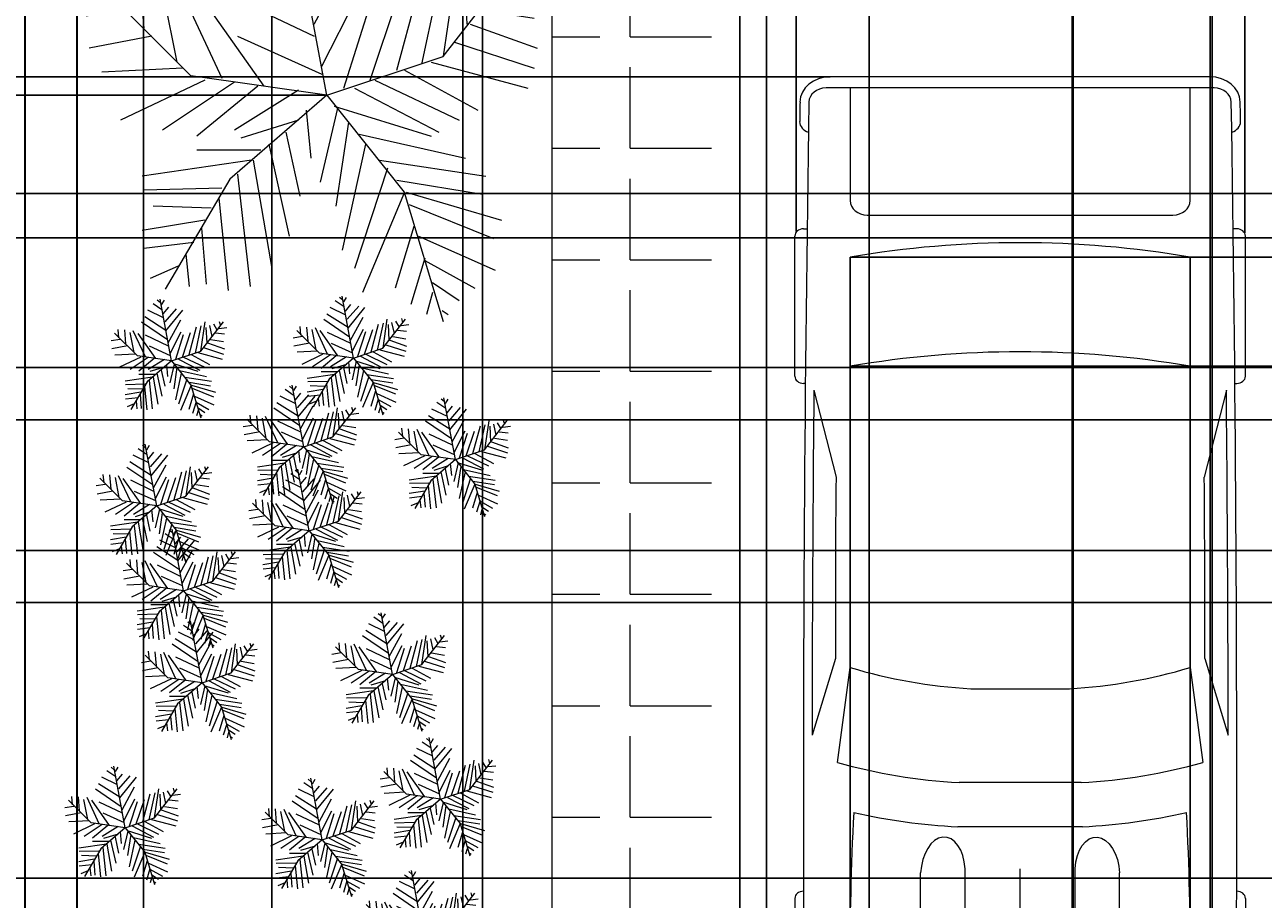
# Model space of a CAD drawing. Units: inches. Extents: x 818 to 1898, y 976 to 2364.
# Tile 4 of 96: x 993 to 1207, y 1295 to 1446. Entities that reach past the tile are written whole.
import ezdxf

# ---------------------------------------------------------------- set-up
doc = ezdxf.new("R2010")
doc.units = ezdxf.units.IN
doc.header["$LTSCALE"] = 5
doc.header["$MEASUREMENT"] = 0
for name, color, linetype, lineweight in [('A-ANNO-DIMS', 2, 'Continuous', 18), ('C-PKNG', 8, 'Continuous', 18), ('C-PKNG-PATT', 9, 'Continuous', 9), ('C-PROP', 7, 'Continuous', 35), ('L-PLNT-BEDS', 94, 'Continuous', 18)]:
    doc.layers.add(name, color=color, linetype=linetype, lineweight=lineweight)
doc.layers.add('L-PLNT', color=116, linetype='Continuous', lineweight=13, true_color=0x136734)
doc.styles.get("Standard").update_dxf_attribs({"font": 'arial.ttf'})
doc.dimstyles.get("Standard").update_dxf_attribs({"dimtxt": 0.18, "dimasz": 0.18, "dimexe": 0.18, "dimexo": 0.0625, "dimgap": 0.09, "dimtad": 0, "dimtih": 1, "dimtoh": 1, "dimdec": 4, "dimzin": 0, "dimdsep": 46, "dimtxsty": 'Standard', "dimcen": 0.09, "dimadec": 0, "dimazin": 0, "dimtfac": 1, "dimtdec": 4, "dimtofl": 0, "dimtmove": 0, "dimatfit": 3, "dimfxl": 1, "dimtolj": 1, "dimtzin": 0, "dimarcsym": 0})
pattern_1 = [(0, (0, 0), (0, 19.25), [14, -5.25]), (90, (0, 0), (-19.25, 1e-15), [14, -5.25])]

# ---------------------------------------------------------------- blocks, each defined once
blk = doc.blocks.new('*U13')
for p, q in [((46.55, 38.89), (22.35, 38.89)), ((136.7, 38.89), (160.9, 38.89)), ((47.8, 37.39), (47.8, 37.41)), ((135.45, 37.07), (135.45, 37.41)), ((162.15, 37.41), (162.15, 36.77)), ((87.99, 31.87), (74.76, 35.92)), ((134.31, 35.6), (119.29, 31.78)), ((186.47, -33.5), (186.47, 33.5)), ((188.4, -32.76), (188.4, 32.76)), ((70.03, 31.54), (86.41, 29.35)), ((138.42, 29.35), (157.25, 29.35)), ((186.47, 29.35), (167.01, 29.35)), ((164.52, 26.39), (164.52, -26.39)), ((36.13, 17.17), (50.94, 17.17)), ((58.92, -10.77), (58.92, 10.77)), ((29.77, 9.51), (51.68, 9.51)), ((66.55, -10.53), (66.55, 10.53)), ((186.47, -10.53), (186.47, 10.53)), ((82.74, 8.5), (82.74, -8.5)), ((0, 0), (51.68, 0)), ((29.77, -9.51), (51.68, -9.51)), ((36.13, -17.17), (50.94, -17.17)), ((86.41, -29.35), (70.03, -31.54)), ((157.25, -29.35), (138.42, -29.35)), ((167.01, -29.35), (186.47, -29.35)), ((87.99, -31.87), (74.76, -35.92)), ((134.31, -35.6), (119.29, -31.78)), ((47.8, -37.39), (47.8, -37.41)), ((135.45, -37.07), (135.45, -37.41)), ((162.15, -37.41), (162.15, -36.77)), ((46.55, -38.89), (22.35, -38.89)), ((136.7, -38.89), (160.9, -38.89))]:
    blk.add_line(p, q)
for centre, major_axis, ratio, start_param, end_param in [((46.55, 37.41), (0, 1.48), 0.842304, -1.570796, 0), ((136.7, 37.41), (0, -1.48), 0.842304, 3.141593, 4.712389), ((160.9, 37.41), (0, 1.48), 0.842304, -1.570796, 0), ((64.48, -10555.62), (0, 10593.03), 0.842304, -0.013397, 0.002797), ((180.63, 35.84), (0, 2.22), 0.842304, -0.013017, 1.249894), ((64.48, -10556.36), (0, 10595.31), 0.842304, -0.013397, -0.013017), ((183.98, 33.5), (0, -2.96), 0.842304, 1.570796, 3.128196), ((183.98, 32.76), (0, -5.25), 0.842304, 1.570796, 3.128196), ((64.48, -10555.62), (0, -10591.55), 0.842304, 3.133765, 3.140441), ((135.29, 5.39), (0, 81.77), 0.842304, 1.245306, 1.50788), ((95.79, -3666.35), (0, -3698.24), 0.842304, 3.134049, 3.144098), ((37.47, -593.96), (0, -623.33), 0.842304, 3.096046, 3.200911), ((134.4, 5.39), (0, -89.78), 0.842304, 4.449482, 4.652344), ((149.6, 2.8), (0, -79.58), 0.842304, 4.372215, 4.640744), ((17.08, 0), (0, 147.02), 0.842304, 4.511394, 4.913384), ((35.91, 0), (0, 147.02), 0.842304, 4.511394, 4.913384), ((167.01, 26.39), (0, 2.96), 0.842304, 0, 1.570796), ((50.79, 13.34), (6.34, -0.36), 0.603834, -1.395552, 1.581315), ((149.6, -2.8), (0, -79.58), 0.842304, -1.499151, -1.230623), ((135.29, -5.39), (0, -81.77), 0.842304, -1.50788, -1.245306), ((134.4, -5.39), (0, -89.78), 0.842304, -1.510751, -1.307889), ((167.01, -26.39), (0, -2.96), 0.842304, 4.712389, 6.283185), ((37.47, 593.96), (0, -623.33), 0.842304, -0.059319, 0.045547), ((95.79, 3666.35), (0, -3698.24), 0.842304, -0.002505, 0.007544), ((183.98, -33.5), (0, 2.96), 0.842304, 3.15499, 4.712389), ((183.98, -32.76), (0, -5.25), 0.842304, 0.013397, 1.570796), ((64.48, 10555.62), (0, -10591.55), 0.842304, 0.001152, 0.007828), ((64.48, 10555.62), (0, 10593.03), 0.842304, 3.138796, 3.15499), ((46.55, -37.41), (0, -1.48), 0.842304, 0, 1.570796), ((136.7, -37.41), (0, -1.48), 0.842304, -1.570796, 0), ((160.9, -37.41), (0, 1.48), 0.842304, 3.141593, 4.712389), ((180.63, -35.84), (0, -2.22), 0.842304, -1.249894, 0.013017), ((64.48, 10556.36), (0, 10595.31), 0.842304, 3.15461, 3.15499)]:
    blk.add_ellipse(centre, major_axis=major_axis, ratio=ratio, start_param=start_param, end_param=end_param)
at = {"extrusion": (0, 0, -1)}
blk.add_ellipse((50.79, -13.34), major_axis=(6.34, 0.36), ratio=0.603834, start_param=-1.395552, end_param=1.581315, dxfattribs=at)
blk = doc.blocks.new('SHRUB-ACCENT')
for p, q in [((8.8, 18.63), (7.25, 19.67)), ((8.53, 19.84), (7.99, 20.28)), ((10.44, 9.82), (8.47, 20.47)), ((8.74, 19.5), (9.21, 20.28)), ((9.48, 15.07), (5.82, 17.41)), ((9.08, 17.24), (6.37, 18.54)), ((9.01, 17.93), (9.96, 19.06)), ((9.35, 16.54), (11.31, 18.8)), ((9.48, 14.98), (12.39, 18.54)), ((1.35, 13.77), (1.22, 15.24)), ((2.3, 15.16), (2.51, 12.72)), ((3.79, 15.07), (5.89, 10.55)), ((9.75, 13.42), (5.28, 16.46)), ((9.89, 12.9), (12.06, 16.89)), ((13.48, 10.9), (14.76, 15.68)), ((14.56, 11.16), (15.58, 15.85)), ((15.49, 11.5), (19.41, 16.55)), ((15.51, 11.51), (16.25, 16.54)), ((16.39, 15.59), (16.53, 12.9)), ((17, 15.94), (17.41, 14.03)), ((17.68, 16.2), (18.29, 15.16)), ((18.62, 15.42), (19.98, 15.59)), ((18.69, 16.63), (18.9, 15.94)), ((1.56, 13.51), (0, 13.25)), ((4.55, 10.66), (0.62, 14.58)), ((3.25, 14.72), (3.93, 11.25)), ((7.72, 10.21), (4.67, 14.55)), ((5.89, 14.29), (9.89, 12.38)), ((10.23, 11.07), (12.12, 14.81)), ((11.17, 10.12), (12.53, 14.37)), ((12.33, 10.47), (13.75, 14.72)), ((16.66, 12.9), (19.57, 11.86)), ((17.2, 13.51), (19.44, 13.16)), ((18.02, 14.63), (19.57, 14.46)), ((2.84, 12.38), (0.14, 11.86)), ((4.2, 10.99), (0.68, 10.81)), ((6.57, 12.38), (10.23, 10.73)), ((10.44, 9.82), (15.49, 11.5)), ((13.82, 10.9), (17, 9.16)), ((14.97, 11.25), (19.17, 10.12)), ((15.98, 12.12), (19.44, 10.99)), ((5.15, 10.47), (1.49, 8.73)), ((6.43, 10.38), (3.32, 8.3)), ((10.44, 9.82), (4.55, 10.66)), ((7.45, 10.21), (4.81, 8.04)), ((10.44, 9.82), (6.23, 6.17)), ((9.21, 10.03), (6.43, 8.3)), ((9.21, 8.73), (6.7, 7.95)), ((9.55, 9.16), (9.75, 7.08)), ((10.9, 9.25), (10.16, 6.04)), ((10.44, 9.82), (13.8, 5.61)), ((10.77, 9.34), (14.97, 8.04)), ((11.38, 8.64), (10.84, 5)), ((11.65, 10.12), (15.31, 8.21)), ((12.53, 10.47), (16.19, 8.73)), ((7.18, 6.99), (2.44, 6.3)), ((7.59, 7.43), (4.81, 7.43)), ((7.25, 6.99), (8.06, 2.31)), ((7.92, 7.69), (8.8, 3.69)), ((8.67, 8.21), (9.28, 5.43)), ((12.12, 7.69), (11.11, 3.09)), ((13.07, 6.65), (11.65, 2.31)), ((11.85, 8.12), (16.46, 7.08)), ((12.73, 6.99), (17.34, 6.3)), ((5.15, 4.39), (2.44, 3.95)), ((5.89, 5.78), (2.51, 5.69)), ((5.42, 4.91), (2.91, 5)), ((6.23, 6.17), (3.43, 1.4)), ((5.76, 5.34), (6.16, 1.35)), ((6.57, 6.39), (7.11, 1.52)), ((13.82, 5.6), (11.99, 1.26)), ((13.48, 6.13), (17.2, 5.52)), ((13.8, 5.61), (15.49, 0)), ((13.88, 5.6), (18.02, 4.39)), ((14.02, 5.08), (17.68, 3.61)), ((4.67, 3.43), (2.51, 3.17)), ((4, 2.39), (2.78, 1.87)), ((4.33, 2.91), (4.47, 1.52)), ((5.01, 4.04), (5.21, 1.61)), ((14.22, 4.13), (13.41, 1.44)), ((14.7, 2.74), (14.09, 0.74)), ((14.43, 3.69), (17.74, 2.22)), ((14.7, 2.65), (16.86, 1.44)), ((15.04, 1.26), (14.76, 0.31)), ((15.04, 1.7), (16.19, 0.92)), ((15.44, 0.48), (15.71, 0.31))]:
    blk.add_line(p, q)
blk = doc.blocks.new('PALM-BORDER')
for p, q in [((41.53, 39.05), (33.72, 81.45)), ((33.95, 78.95), (31.8, 80.68)), ((34.76, 77.57), (36.65, 80.68)), ((35.03, 74.11), (28.83, 78.26)), ((35.84, 71.35), (39.61, 75.84)), ((36.11, 68.59), (25.33, 73.77)), ((37.18, 65.82), (45, 74.8)), ((37.72, 59.6), (49.31, 73.77)), ((37.72, 59.95), (23.17, 69.28)), ((39.34, 51.31), (47.96, 67.2)), ((38.8, 53.39), (21.02, 65.48)), ((61.61, 45.75), (77.23, 65.83)), ((61.71, 45.79), (64.67, 65.82)), ((70.33, 64.44), (72.75, 60.3)), ((74.37, 66.17), (75.18, 63.4)), ((53.62, 43.37), (58.74, 62.37)), ((57.93, 44.41), (61.97, 63.06)), ((65.21, 62.02), (65.75, 51.31)), ((67.63, 63.4), (69.25, 55.81)), ((74.1, 61.33), (79.49, 62.02)), ((5.39, 54.77), (4.85, 60.64)), ((9.16, 60.3), (9.97, 50.62)), ((15.09, 59.95), (23.44, 41.99)), ((18.1, 42.4), (2.48, 58.02)), ((12.93, 58.57), (15.63, 44.75)), ((30.72, 40.61), (18.59, 57.88)), ((40.69, 44.06), (48.23, 58.91)), ((49.04, 41.64), (54.7, 58.57)), ((71.68, 58.22), (77.87, 57.53)), ((23.44, 56.84), (39.34, 49.24)), ((44.46, 40.26), (49.85, 57.19)), ((6.2, 53.73), (0, 52.7)), ((68.44, 53.73), (77.33, 52.35)), ((66.29, 51.31), (77.87, 47.17)), ((11.32, 49.24), (0.54, 47.17)), ((26.14, 49.24), (40.69, 42.68)), ((63.59, 48.21), (77.33, 43.71)), ((41.53, 39.05), (61.61, 45.75)), ((16.71, 43.71), (2.69, 43.02)), ((54.97, 43.37), (67.63, 36.46)), ((59.55, 44.75), (76.26, 40.26)), ((20.48, 41.64), (5.93, 34.73)), ((25.6, 41.3), (13.2, 33.01)), ((41.53, 39.05), (18.1, 42.4)), ((49.85, 41.64), (64.4, 34.73)), ((29.64, 40.61), (19.13, 31.97)), ((41.53, 39.05), (24.79, 24.55)), ((36.65, 39.91), (25.6, 33.01)), ((41.53, 39.05), (54.92, 22.32)), ((46.35, 40.26), (60.9, 32.66)), ((37.99, 36.46), (38.8, 28.17)), ((43.38, 36.81), (40.42, 24.02)), ((42.84, 37.15), (59.55, 31.97)), ((36.65, 34.73), (26.68, 31.62)), ((45.27, 34.39), (43.11, 19.88)), ((34.49, 32.66), (36.92, 21.61)), ((47.15, 32.32), (65.48, 28.17)), ((31.53, 30.59), (35.03, 14.7)), ((48.23, 30.59), (44.19, 12.28)), ((28.56, 27.82), (9.7, 25.06)), ((30.18, 29.55), (19.13, 29.55)), ((28.83, 27.82), (32.07, 9.17)), ((50.66, 27.82), (68.98, 25.06)), ((52, 26.44), (46.35, 9.17)), ((24.79, 24.55), (13.63, 5.58)), ((26.14, 25.41), (28.29, 6.06)), ((53.62, 24.37), (68.44, 21.95)), ((23.44, 22.99), (9.97, 22.64)), ((54.97, 22.3), (47.69, 5.02)), ((54.92, 22.32), (61.61, 0)), ((55.24, 22.3), (71.68, 17.46)), ((21.56, 19.53), (11.59, 19.88)), ((22.9, 21.26), (24.52, 5.37)), ((55.78, 20.22), (70.33, 14.35)), ((20.48, 17.46), (9.7, 15.73)), ((19.94, 16.08), (20.75, 6.41)), ((56.59, 16.42), (53.35, 5.72)), ((18.59, 13.66), (9.97, 12.62)), ((57.39, 14.7), (70.6, 8.83)), ((17.24, 11.59), (17.78, 6.06)), ((58.47, 10.9), (56.05, 2.95)), ((15.9, 9.52), (11.05, 7.44)), ((58.47, 10.55), (67.09, 5.72)), ((59.82, 6.75), (64.4, 3.64)), ((59.82, 5.02), (58.74, 1.22)), ((61.44, 1.92), (62.51, 1.22))]:
    blk.add_line(p, q)
blk = doc.blocks.new('*D59')
at = {"layer": 'A-ANNO-DIMS', "color": 0, "lineweight": -2, "ltscale": 5, "transparency": 16777216}
for p, q in [((1251.64, 2300.39), (818.03, 2300.39)), ((818.21, 2300.21), (818.21, 1669.95)), ((818.21, 1039.32), (818.21, 1669.59)), ((896.05, 1039.14), (818.03, 1039.14))]:
    blk.add_line(p, q, dxfattribs=at)
at = {"layer": 'A-ANNO-DIMS', "color": 0, "ltscale": 5, "transparency": 16777216}
for points in [[(818.18, 2300.21), (818.24, 2300.21), (818.21, 2300.39)], [(818.18, 1039.32), (818.24, 1039.32), (818.21, 1039.14)]]:
    blk.add_solid(points, dxfattribs=at)
at = {"layer": 'Defpoints', "color": 0, "ltscale": 5, "transparency": 16777216}
for p in [(818.21, 2300.39), (1251.71, 2300.39), (896.11, 1039.14)]:
    blk.add_point(p, dxfattribs=at)
at = {"layer": 'A-ANNO-DIMS', "color": 0, "ltscale": 5, "transparency": 16777216, "insert": (818.21, 1669.77), "char_height": 0.18, "attachment_point": 5}
blk.add_mtext('\\A1;1261.2', dxfattribs=at)
blk = doc.blocks.new('*D61')
at = {"layer": 'A-ANNO-DIMS', "color": 0, "lineweight": -2, "ltscale": 5, "transparency": 16777216}
for p, q in [((1071.73, 1203.03), (1071.73, 2363.87)), ((1071.91, 2363.69), (1250.94, 2363.69)), ((1430.55, 2363.69), (1251.51, 2363.69)), ((1430.73, 1203.03), (1430.73, 2363.87))]:
    blk.add_line(p, q, dxfattribs=at)
at = {"layer": 'A-ANNO-DIMS', "color": 0, "ltscale": 5, "transparency": 16777216}
for points in [[(1071.91, 2363.72), (1071.91, 2363.66), (1071.73, 2363.69)], [(1430.55, 2363.72), (1430.55, 2363.66), (1430.73, 2363.69)]]:
    blk.add_solid(points, dxfattribs=at)
at = {"layer": 'Defpoints', "color": 0, "ltscale": 5, "transparency": 16777216}
for p in [(1430.73, 2363.69), (1071.73, 1202.96), (1430.73, 1202.96)]:
    blk.add_point(p, dxfattribs=at)
at = {"layer": 'A-ANNO-DIMS', "color": 0, "ltscale": 5, "transparency": 16777216, "insert": (1251.23, 2363.69), "char_height": 0.18, "attachment_point": 5}
blk.add_mtext('\\A1;359', dxfattribs=at)
blk = doc.blocks.new('*D63')
at = {"layer": 'A-ANNO-DIMS', "color": 0, "lineweight": -2, "ltscale": 5, "transparency": 16777216}
for p, q in [((1116.13, 1485.2), (818.03, 1485.2)), ((818.21, 1485.02), (818.21, 1360.77)), ((818.21, 1236.14), (818.21, 1360.4)), ((1116.13, 1235.96), (818.03, 1235.96))]:
    blk.add_line(p, q, dxfattribs=at)
at = {"layer": 'A-ANNO-DIMS', "color": 0, "ltscale": 5, "transparency": 16777216}
for points in [[(818.18, 1485.02), (818.24, 1485.02), (818.21, 1485.2)], [(818.18, 1236.14), (818.24, 1236.14), (818.21, 1235.96)]]:
    blk.add_solid(points, dxfattribs=at)
at = {"layer": 'Defpoints', "color": 0, "ltscale": 5, "transparency": 16777216}
for p in [(818.21, 1485.2), (1116.19, 1485.2), (1116.19, 1235.96)]:
    blk.add_point(p, dxfattribs=at)
at = {"layer": 'A-ANNO-DIMS', "color": 0, "ltscale": 5, "transparency": 16777216, "insert": (818.21, 1360.58), "char_height": 0.18, "attachment_point": 5}
blk.add_mtext('\\A1;249.24', dxfattribs=at)
blk = doc.blocks.new('*D79')
at = {"layer": 'A-ANNO-DIMS', "color": 0, "lineweight": -2, "ltscale": 5, "transparency": 16777216}
for p, q in [((992.73, 1203.03), (992.73, 2363.87)), ((992.91, 2363.69), (1032.01, 2363.69)), ((1071.55, 2363.69), (1032.44, 2363.69)), ((1071.73, 1203.03), (1071.73, 2363.87))]:
    blk.add_line(p, q, dxfattribs=at)
at = {"layer": 'A-ANNO-DIMS', "color": 0, "ltscale": 5, "transparency": 16777216}
for points in [[(992.91, 2363.72), (992.91, 2363.66), (992.73, 2363.69)], [(1071.55, 2363.72), (1071.55, 2363.66), (1071.73, 2363.69)]]:
    blk.add_solid(points, dxfattribs=at)
at = {"layer": 'Defpoints', "color": 0, "ltscale": 5, "transparency": 16777216}
for p in [(1071.73, 2363.69), (992.73, 1202.96), (1071.73, 1202.96)]:
    blk.add_point(p, dxfattribs=at)
at = {"layer": 'A-ANNO-DIMS', "color": 0, "ltscale": 5, "transparency": 16777216, "insert": (1032.23, 2363.69), "char_height": 0.18, "attachment_point": 5}
blk.add_mtext('\\A1;79', dxfattribs=at)
blk = doc.blocks.new('*D91')
at = {"layer": 'A-ANNO-DIMS', "color": 0, "lineweight": -2, "ltscale": 5, "transparency": 16777216}
for p, q in [((959.17, 1071.12), (959.17, 2363.87)), ((959.35, 2363.69), (985.8, 2363.69)), ((1013.04, 2363.69), (986.59, 2363.69)), ((1013.22, 1071.12), (1013.22, 2363.87))]:
    blk.add_line(p, q, dxfattribs=at)
at = {"layer": 'A-ANNO-DIMS', "color": 0, "ltscale": 5, "transparency": 16777216}
for points in [[(959.35, 2363.72), (959.35, 2363.66), (959.17, 2363.69)], [(1013.04, 2363.72), (1013.04, 2363.66), (1013.22, 2363.69)]]:
    blk.add_solid(points, dxfattribs=at)
at = {"layer": 'Defpoints', "color": 0, "ltscale": 5, "transparency": 16777216}
for p in [(1013.22, 2363.69), (959.17, 1071.06), (1013.22, 1071.06)]:
    blk.add_point(p, dxfattribs=at)
at = {"layer": 'A-ANNO-DIMS', "color": 0, "ltscale": 5, "transparency": 16777216, "insert": (986.2, 2363.69), "char_height": 0.18, "attachment_point": 5}
blk.add_mtext('\\A1;54.04', dxfattribs=at)
blk = doc.blocks.new('*D92')
at = {"layer": 'A-ANNO-DIMS', "color": 0, "lineweight": -2, "ltscale": 5, "transparency": 16777216}
for p, q in [((1013.22, 1071.12), (1013.22, 2363.87)), ((1013.4, 2363.69), (1040.38, 2363.69)), ((1068.16, 2363.69), (1041.17, 2363.69)), ((1068.34, 1071.12), (1068.34, 2363.87))]:
    blk.add_line(p, q, dxfattribs=at)
at = {"layer": 'A-ANNO-DIMS', "color": 0, "ltscale": 5, "transparency": 16777216}
for points in [[(1013.4, 2363.72), (1013.4, 2363.66), (1013.22, 2363.69)], [(1068.16, 2363.72), (1068.16, 2363.66), (1068.34, 2363.69)]]:
    blk.add_solid(points, dxfattribs=at)
at = {"layer": 'Defpoints', "color": 0, "ltscale": 5, "transparency": 16777216}
for p in [(1068.34, 2363.69), (1013.22, 1071.06), (1068.34, 1071.06)]:
    blk.add_point(p, dxfattribs=at)
at = {"layer": 'A-ANNO-DIMS', "color": 0, "ltscale": 5, "transparency": 16777216, "insert": (1040.78, 2363.69), "char_height": 0.18, "attachment_point": 5}
blk.add_mtext('\\A1;55.12', dxfattribs=at)
blk = doc.blocks.new('*D93')
at = {"layer": 'A-ANNO-DIMS', "color": 0, "lineweight": -2, "ltscale": 5, "transparency": 16777216}
for p, q in [((1068.34, 1071.12), (1068.34, 2363.87)), ((1068.52, 2363.69), (1094.16, 2363.69)), ((1120.58, 2363.69), (1094.94, 2363.69)), ((1120.76, 1071.12), (1120.76, 2363.87))]:
    blk.add_line(p, q, dxfattribs=at)
at = {"layer": 'A-ANNO-DIMS', "color": 0, "ltscale": 5, "transparency": 16777216}
for points in [[(1068.52, 2363.72), (1068.52, 2363.66), (1068.34, 2363.69)], [(1120.58, 2363.72), (1120.58, 2363.66), (1120.76, 2363.69)]]:
    blk.add_solid(points, dxfattribs=at)
at = {"layer": 'Defpoints', "color": 0, "ltscale": 5, "transparency": 16777216}
for p in [(1120.76, 2363.69), (1068.34, 1071.06), (1120.76, 1071.06)]:
    blk.add_point(p, dxfattribs=at)
at = {"layer": 'A-ANNO-DIMS', "color": 0, "ltscale": 5, "transparency": 16777216, "insert": (1094.55, 2363.69), "char_height": 0.18, "attachment_point": 5}
blk.add_mtext('\\A1;52.42', dxfattribs=at)
blk = doc.blocks.new('*D94')
at = {"layer": 'A-ANNO-DIMS', "color": 0, "lineweight": -2, "ltscale": 5, "transparency": 16777216}
for p, q in [((1120.76, 1071.12), (1120.76, 2363.87)), ((1120.94, 2363.69), (1146.76, 2363.69)), ((1173.36, 2363.69), (1147.55, 2363.69)), ((1173.54, 1071.12), (1173.54, 2363.87))]:
    blk.add_line(p, q, dxfattribs=at)
at = {"layer": 'A-ANNO-DIMS', "color": 0, "ltscale": 5, "transparency": 16777216}
for points in [[(1120.94, 2363.72), (1120.94, 2363.66), (1120.76, 2363.69)], [(1173.36, 2363.72), (1173.36, 2363.66), (1173.54, 2363.69)]]:
    blk.add_solid(points, dxfattribs=at)
at = {"layer": 'Defpoints', "color": 0, "ltscale": 5, "transparency": 16777216}
for p in [(1173.54, 2363.69), (1120.76, 1071.06), (1173.54, 1071.06)]:
    blk.add_point(p, dxfattribs=at)
at = {"layer": 'A-ANNO-DIMS', "color": 0, "ltscale": 5, "transparency": 16777216, "insert": (1147.15, 2363.69), "char_height": 0.18, "attachment_point": 5}
blk.add_mtext('\\A1;52.78', dxfattribs=at)
blk = doc.blocks.new('*D95')
at = {"layer": 'A-ANNO-DIMS', "color": 0, "lineweight": -2, "ltscale": 5, "transparency": 16777216}
for p, q in [((1173.54, 1071.12), (1173.54, 2363.87)), ((1173.72, 2363.69), (1201.29, 2363.69)), ((1229.47, 2363.69), (1201.9, 2363.69)), ((1229.65, 1071.12), (1229.65, 2363.87))]:
    blk.add_line(p, q, dxfattribs=at)
at = {"layer": 'A-ANNO-DIMS', "color": 0, "ltscale": 5, "transparency": 16777216}
for points in [[(1173.72, 2363.72), (1173.72, 2363.66), (1173.54, 2363.69)], [(1229.47, 2363.72), (1229.47, 2363.66), (1229.65, 2363.69)]]:
    blk.add_solid(points, dxfattribs=at)
at = {"layer": 'Defpoints', "color": 0, "ltscale": 5, "transparency": 16777216}
for p in [(1229.65, 2363.69), (1173.54, 1071.06), (1229.65, 1071.06)]:
    blk.add_point(p, dxfattribs=at)
at = {"layer": 'A-ANNO-DIMS', "color": 0, "ltscale": 5, "transparency": 16777216, "insert": (1201.59, 2363.69), "char_height": 0.18, "attachment_point": 5}
blk.add_mtext('\\A1;56.1', dxfattribs=at)
blk = doc.blocks.new('*D108')
at = {"layer": 'A-ANNO-DIMS', "color": 0, "lineweight": -2, "ltscale": 5, "transparency": 16777216}
for p, q in [((1131.74, 1436.86), (818.03, 1436.86)), ((818.21, 1436.68), (818.21, 1342.84)), ((818.21, 1248.64), (818.21, 1342.48)), ((1164.49, 1248.46), (818.03, 1248.46))]:
    blk.add_line(p, q, dxfattribs=at)
at = {"layer": 'A-ANNO-DIMS', "color": 0, "ltscale": 5, "transparency": 16777216}
for points in [[(818.18, 1436.68), (818.24, 1436.68), (818.21, 1436.86)], [(818.18, 1248.64), (818.24, 1248.64), (818.21, 1248.46)]]:
    blk.add_solid(points, dxfattribs=at)
at = {"layer": 'Defpoints', "color": 0, "ltscale": 5, "transparency": 16777216}
for p in [(818.21, 1436.86), (1131.8, 1436.86), (1164.56, 1248.46)]:
    blk.add_point(p, dxfattribs=at)
at = {"layer": 'A-ANNO-DIMS', "color": 0, "ltscale": 5, "transparency": 16777216, "insert": (818.21, 1342.66), "char_height": 0.18, "attachment_point": 5}
blk.add_mtext('\\A1;188.4', dxfattribs=at)
blk = doc.blocks.new('*D109')
at = {"layer": 'A-ANNO-DIMS', "color": 0, "lineweight": -2, "ltscale": 5, "transparency": 16777216}
for p, q in [((1125.92, 1410.12), (1125.92, 2363.87)), ((1126.1, 2363.69), (1164.25, 2363.69)), ((1203.15, 2363.69), (1165, 2363.69)), ((1203.33, 1409.91), (1203.33, 2363.87))]:
    blk.add_line(p, q, dxfattribs=at)
at = {"layer": 'A-ANNO-DIMS', "color": 0, "ltscale": 5, "transparency": 16777216}
for points in [[(1126.1, 2363.72), (1126.1, 2363.66), (1125.92, 2363.69)], [(1203.15, 2363.72), (1203.15, 2363.66), (1203.33, 2363.69)]]:
    blk.add_solid(points, dxfattribs=at)
at = {"layer": 'Defpoints', "color": 0, "ltscale": 5, "transparency": 16777216}
for p in [(1203.33, 2363.69), (1125.92, 1410.05), (1203.33, 1409.85)]:
    blk.add_point(p, dxfattribs=at)
at = {"layer": 'A-ANNO-DIMS', "color": 0, "ltscale": 5, "transparency": 16777216, "insert": (1164.62, 2363.69), "char_height": 0.18, "attachment_point": 5}
blk.add_mtext('\\A1;77.41', dxfattribs=at)
blk = doc.blocks.new('*D111')
at = {"layer": 'A-ANNO-DIMS', "color": 0, "lineweight": -2, "ltscale": 5, "transparency": 16777216}
for p, q in [((1135.21, 1405.65), (1135.21, 975.66)), ((1193.91, 1405.65), (1193.91, 975.66)), ((1135.39, 975.84), (1164.23, 975.84)), ((1193.73, 975.84), (1164.88, 975.84))]:
    blk.add_line(p, q, dxfattribs=at)
at = {"layer": 'A-ANNO-DIMS', "color": 0, "ltscale": 5, "transparency": 16777216}
for points in [[(1135.39, 975.87), (1135.39, 975.81), (1135.21, 975.84)], [(1193.73, 975.87), (1193.73, 975.81), (1193.91, 975.84)]]:
    blk.add_solid(points, dxfattribs=at)
at = {"layer": 'Defpoints', "color": 0, "ltscale": 5, "transparency": 16777216}
for p in [(1135.21, 1405.71), (1193.91, 1405.71), (1193.91, 975.84)]:
    blk.add_point(p, dxfattribs=at)
at = {"layer": 'A-ANNO-DIMS', "color": 0, "ltscale": 5, "transparency": 16777216, "insert": (1164.56, 975.84), "char_height": 0.18, "attachment_point": 5}
blk.add_mtext('\\A1;58.7', dxfattribs=at)
blk = doc.blocks.new('*D112')
at = {"layer": 'A-ANNO-DIMS', "color": 0, "lineweight": -2, "ltscale": 5, "transparency": 16777216}
for p, q in [((1135.27, 1405.71), (1897.92, 1405.71)), ((1897.74, 1405.53), (1897.74, 1396.48)), ((1897.74, 1387.07), (1897.74, 1396.12)), ((1135.27, 1386.89), (1897.92, 1386.89))]:
    blk.add_line(p, q, dxfattribs=at)
at = {"layer": 'A-ANNO-DIMS', "color": 0, "ltscale": 5, "transparency": 16777216}
for points in [[(1897.71, 1405.53), (1897.77, 1405.53), (1897.74, 1405.71)], [(1897.71, 1387.07), (1897.77, 1387.07), (1897.74, 1386.89)]]:
    blk.add_solid(points, dxfattribs=at)
at = {"layer": 'Defpoints', "color": 0, "ltscale": 5, "transparency": 16777216}
for p in [(1135.21, 1405.71), (1135.21, 1386.89), (1897.74, 1386.89)]:
    blk.add_point(p, dxfattribs=at)
at = {"layer": 'A-ANNO-DIMS', "color": 0, "ltscale": 5, "transparency": 16777216, "insert": (1897.74, 1396.3), "char_height": 0.18, "attachment_point": 5}
blk.add_mtext('\\A1;18.824', dxfattribs=at)
blk = doc.blocks.new('*D115')
at = {"layer": 'A-ANNO-DIMS', "color": 0, "lineweight": -2, "ltscale": 5, "transparency": 16777216}
for p, q in [((1766.29, 1377.66), (818.03, 1377.66)), ((818.21, 1377.48), (818.21, 1338.26)), ((818.21, 1298.68), (818.21, 1337.9)), ((1766.29, 1298.5), (818.03, 1298.5))]:
    blk.add_line(p, q, dxfattribs=at)
at = {"layer": 'A-ANNO-DIMS', "color": 0, "ltscale": 5, "transparency": 16777216}
for points in [[(818.18, 1377.48), (818.24, 1377.48), (818.21, 1377.66)], [(818.18, 1298.68), (818.24, 1298.68), (818.21, 1298.5)]]:
    blk.add_solid(points, dxfattribs=at)
at = {"layer": 'Defpoints', "color": 0, "ltscale": 5, "transparency": 16777216}
for p in [(818.21, 1377.66), (1766.35, 1377.66), (1766.35, 1298.5)]:
    blk.add_point(p, dxfattribs=at)
at = {"layer": 'A-ANNO-DIMS', "color": 0, "ltscale": 5, "transparency": 16777216, "insert": (818.21, 1338.08), "char_height": 0.18, "attachment_point": 5}
blk.add_mtext('\\A1;79.15', dxfattribs=at)
blk = doc.blocks.new('*D116')
at = {"layer": 'A-ANNO-DIMS', "color": 0, "lineweight": -2, "ltscale": 5, "transparency": 16777216}
for p, q in [((1766.29, 1456.81), (818.03, 1456.81)), ((818.21, 1456.63), (818.21, 1417.41)), ((818.21, 1377.84), (818.21, 1417.05)), ((1766.29, 1377.66), (818.03, 1377.66))]:
    blk.add_line(p, q, dxfattribs=at)
at = {"layer": 'A-ANNO-DIMS', "color": 0, "ltscale": 5, "transparency": 16777216}
for points in [[(818.18, 1456.63), (818.24, 1456.63), (818.21, 1456.81)], [(818.18, 1377.84), (818.24, 1377.84), (818.21, 1377.66)]]:
    blk.add_solid(points, dxfattribs=at)
at = {"layer": 'Defpoints', "color": 0, "ltscale": 5, "transparency": 16777216}
for p in [(818.21, 1456.81), (1766.35, 1456.81), (1766.35, 1377.66)]:
    blk.add_point(p, dxfattribs=at)
at = {"layer": 'A-ANNO-DIMS', "color": 0, "ltscale": 5, "transparency": 16777216, "insert": (818.21, 1417.23), "char_height": 0.18, "attachment_point": 5}
blk.add_mtext('\\A1;79.15', dxfattribs=at)
blk = doc.blocks.new('*D122')
at = {"layer": 'A-ANNO-DIMS', "color": 0, "lineweight": -2, "ltscale": 5, "transparency": 16777216}
for p, q in [((1138.5, 1794.37), (1138.5, 975.66)), ((1071.73, 1688.02), (1071.73, 975.66)), ((1071.91, 975.84), (1104.72, 975.84)), ((1138.32, 975.84), (1105.51, 975.84))]:
    blk.add_line(p, q, dxfattribs=at)
at = {"layer": 'A-ANNO-DIMS', "color": 0, "ltscale": 5, "transparency": 16777216}
for points in [[(1071.91, 975.87), (1071.91, 975.81), (1071.73, 975.84)], [(1138.32, 975.87), (1138.32, 975.81), (1138.5, 975.84)]]:
    blk.add_solid(points, dxfattribs=at)
at = {"layer": 'Defpoints', "color": 0, "ltscale": 5, "transparency": 16777216}
for p in [(1138.5, 1794.43), (1071.73, 1688.08), (1138.5, 975.84)]:
    blk.add_point(p, dxfattribs=at)
at = {"layer": 'A-ANNO-DIMS', "color": 0, "ltscale": 5, "transparency": 16777216, "insert": (1105.11, 975.84), "char_height": 0.18, "attachment_point": 5}
blk.add_mtext('\\A1;66.78', dxfattribs=at)
blk = doc.blocks.new('*D126')
at = {"layer": 'A-ANNO-DIMS', "color": 0, "lineweight": -2, "ltscale": 5, "transparency": 16777216}
for p, q in [((1035.38, 1252.09), (1035.38, 2363.87)), ((1035.56, 2363.69), (1075.41, 2363.69)), ((1116.01, 2363.69), (1076.16, 2363.69)), ((1116.19, 1236.03), (1116.19, 2363.87))]:
    blk.add_line(p, q, dxfattribs=at)
at = {"layer": 'A-ANNO-DIMS', "color": 0, "ltscale": 5, "transparency": 16777216}
for points in [[(1035.56, 2363.72), (1035.56, 2363.66), (1035.38, 2363.69)], [(1116.01, 2363.72), (1116.01, 2363.66), (1116.19, 2363.69)]]:
    blk.add_solid(points, dxfattribs=at)
at = {"layer": 'Defpoints', "color": 0, "ltscale": 5, "transparency": 16777216}
for p in [(1035.38, 2363.69), (1035.38, 1252.02), (1116.19, 1235.96)]:
    blk.add_point(p, dxfattribs=at)
at = {"layer": 'A-ANNO-DIMS', "color": 0, "ltscale": 5, "transparency": 16777216, "insert": (1075.78, 2363.69), "char_height": 0.18, "attachment_point": 5}
blk.add_mtext('\\A1;80.81', dxfattribs=at)
blk = doc.blocks.new('*D128')
at = {"layer": 'A-ANNO-DIMS', "color": 0, "lineweight": -2, "ltscale": 5, "transparency": 16777216}
for p, q in [((1044.78, 1433.67), (818.03, 1433.67)), ((818.21, 1433.49), (818.21, 1343.03)), ((818.21, 1252.2), (818.21, 1342.66)), ((1035.31, 1252.02), (818.03, 1252.02))]:
    blk.add_line(p, q, dxfattribs=at)
at = {"layer": 'A-ANNO-DIMS', "color": 0, "ltscale": 5, "transparency": 16777216}
for points in [[(818.18, 1433.49), (818.24, 1433.49), (818.21, 1433.67)], [(818.18, 1252.2), (818.24, 1252.2), (818.21, 1252.02)]]:
    blk.add_solid(points, dxfattribs=at)
at = {"layer": 'Defpoints', "color": 0, "ltscale": 5, "transparency": 16777216}
for p in [(818.21, 1433.67), (1044.85, 1433.67), (1035.38, 1252.02)]:
    blk.add_point(p, dxfattribs=at)
at = {"layer": 'A-ANNO-DIMS', "color": 0, "ltscale": 5, "transparency": 16777216, "insert": (818.21, 1342.85), "char_height": 0.18, "attachment_point": 5}
blk.add_mtext('\\A1;181.64', dxfattribs=at)
blk = doc.blocks.new('*D129')
at = {"layer": 'A-ANNO-DIMS', "color": 0, "lineweight": -2, "ltscale": 5, "transparency": 16777216}
for p, q in [((1044.78, 1608.51), (818.03, 1608.51)), ((818.21, 1608.33), (818.21, 1521.27)), ((818.21, 1433.85), (818.21, 1520.91)), ((1044.78, 1433.67), (818.03, 1433.67))]:
    blk.add_line(p, q, dxfattribs=at)
at = {"layer": 'A-ANNO-DIMS', "color": 0, "ltscale": 5, "transparency": 16777216}
for points in [[(818.18, 1608.33), (818.24, 1608.33), (818.21, 1608.51)], [(818.18, 1433.85), (818.24, 1433.85), (818.21, 1433.67)]]:
    blk.add_solid(points, dxfattribs=at)
at = {"layer": 'Defpoints', "color": 0, "ltscale": 5, "transparency": 16777216}
for p in [(818.21, 1608.51), (1044.85, 1608.51), (1044.85, 1433.67)]:
    blk.add_point(p, dxfattribs=at)
at = {"layer": 'A-ANNO-DIMS', "color": 0, "ltscale": 5, "transparency": 16777216, "insert": (818.21, 1521.09), "char_height": 0.18, "attachment_point": 5}
blk.add_mtext('\\A1;174.84', dxfattribs=at)
blk = doc.blocks.new('*D145')
at = {"layer": 'A-ANNO-DIMS', "color": 0, "lineweight": -2, "ltscale": 5, "transparency": 16777216}
for p, q in [((1197.39, 2122.31), (1197.39, 975.66)), ((1232.61, 2122.31), (1232.61, 975.66)), ((1197.57, 975.84), (1214.61, 975.84)), ((1232.43, 975.84), (1215.39, 975.84))]:
    blk.add_line(p, q, dxfattribs=at)
at = {"layer": 'A-ANNO-DIMS', "color": 0, "ltscale": 5, "transparency": 16777216}
for points in [[(1197.57, 975.87), (1197.57, 975.81), (1197.39, 975.84)], [(1232.43, 975.87), (1232.43, 975.81), (1232.61, 975.84)]]:
    blk.add_solid(points, dxfattribs=at)
at = {"layer": 'Defpoints', "color": 0, "ltscale": 5, "transparency": 16777216}
for p in [(1197.39, 2122.38), (1232.61, 2122.38), (1232.61, 975.84)]:
    blk.add_point(p, dxfattribs=at)
at = {"layer": 'A-ANNO-DIMS', "color": 0, "ltscale": 5, "transparency": 16777216, "insert": (1215, 975.84), "char_height": 0.18, "attachment_point": 5}
blk.add_mtext('\\A1;35.22', dxfattribs=at)
blk = doc.blocks.new('*D155')
at = {"layer": 'A-ANNO-DIMS', "color": 0, "lineweight": -2, "ltscale": 5, "transparency": 16777216}
for p, q in [((1173.73, 1590.7), (1173.73, 975.66)), ((1197.73, 1530.54), (1197.73, 975.66)), ((1173.91, 975.84), (1185.51, 975.84)), ((1197.55, 975.84), (1185.95, 975.84))]:
    blk.add_line(p, q, dxfattribs=at)
at = {"layer": 'A-ANNO-DIMS', "color": 0, "ltscale": 5, "transparency": 16777216}
for points in [[(1173.91, 975.87), (1173.91, 975.81), (1173.73, 975.84)], [(1197.55, 975.87), (1197.55, 975.81), (1197.73, 975.84)]]:
    blk.add_solid(points, dxfattribs=at)
at = {"layer": 'Defpoints', "color": 0, "ltscale": 5, "transparency": 16777216}
for p in [(1173.73, 1590.76), (1197.73, 1530.6), (1173.73, 975.84)]:
    blk.add_point(p, dxfattribs=at)
at = {"layer": 'A-ANNO-DIMS', "color": 0, "ltscale": 5, "transparency": 16777216, "insert": (1185.73, 975.84), "char_height": 0.18, "attachment_point": 5}
blk.add_mtext('\\A1;24', dxfattribs=at)
blk = doc.blocks.new('*D171')
at = {"layer": 'A-ANNO-DIMS', "color": 0, "lineweight": -2, "ltscale": 5, "transparency": 16777216}
for p, q in [((1616.66, 1386.69), (818.03, 1386.69)), ((818.21, 1386.51), (818.21, 1371.06)), ((818.21, 1355.26), (818.21, 1370.7)), ((1616.66, 1355.08), (818.03, 1355.08))]:
    blk.add_line(p, q, dxfattribs=at)
at = {"layer": 'A-ANNO-DIMS', "color": 0, "ltscale": 5, "transparency": 16777216}
for points in [[(818.18, 1386.51), (818.24, 1386.51), (818.21, 1386.69)], [(818.18, 1355.26), (818.24, 1355.26), (818.21, 1355.08)]]:
    blk.add_solid(points, dxfattribs=at)
at = {"layer": 'Defpoints', "color": 0, "ltscale": 5, "transparency": 16777216}
for p in [(818.21, 1386.69), (1616.73, 1386.69), (1616.73, 1355.08)]:
    blk.add_point(p, dxfattribs=at)
at = {"layer": 'A-ANNO-DIMS', "color": 0, "ltscale": 5, "transparency": 16777216, "insert": (818.21, 1370.88), "char_height": 0.18, "attachment_point": 5}
blk.add_mtext('\\A1;31.61', dxfattribs=at)
blk = doc.blocks.new('*D172')
at = {"layer": 'A-ANNO-DIMS', "color": 0, "lineweight": -2, "ltscale": 5, "transparency": 16777216}
for p, q in [((1616.66, 1416.69), (818.03, 1416.69)), ((818.21, 1416.51), (818.21, 1401.87)), ((818.21, 1386.87), (818.21, 1401.5)), ((1616.66, 1386.69), (818.03, 1386.69))]:
    blk.add_line(p, q, dxfattribs=at)
at = {"layer": 'A-ANNO-DIMS', "color": 0, "ltscale": 5, "transparency": 16777216}
for points in [[(818.18, 1416.51), (818.24, 1416.51), (818.21, 1416.69)], [(818.18, 1386.87), (818.24, 1386.87), (818.21, 1386.69)]]:
    blk.add_solid(points, dxfattribs=at)
at = {"layer": 'Defpoints', "color": 0, "ltscale": 5, "transparency": 16777216}
for p in [(818.21, 1416.69), (1616.73, 1416.69), (1616.73, 1386.69)]:
    blk.add_point(p, dxfattribs=at)
at = {"layer": 'A-ANNO-DIMS', "color": 0, "ltscale": 5, "transparency": 16777216, "insert": (818.21, 1401.69), "char_height": 0.18, "attachment_point": 5}
blk.add_mtext('\\A1;30', dxfattribs=at)
blk = doc.blocks.new('*D190')
at = {"layer": 'A-ANNO-DIMS', "color": 0, "lineweight": -2, "ltscale": 5, "transparency": 16777216}
for p, q in [((1430.66, 1409.05), (818.03, 1409.05)), ((818.21, 1408.87), (818.21, 1377.75)), ((818.21, 1346.26), (818.21, 1377.38)), ((1430.66, 1346.08), (818.03, 1346.08))]:
    blk.add_line(p, q, dxfattribs=at)
at = {"layer": 'A-ANNO-DIMS', "color": 0, "ltscale": 5, "transparency": 16777216}
for points in [[(818.18, 1408.87), (818.24, 1408.87), (818.21, 1409.05)], [(818.18, 1346.26), (818.24, 1346.26), (818.21, 1346.08)]]:
    blk.add_solid(points, dxfattribs=at)
at = {"layer": 'Defpoints', "color": 0, "ltscale": 5, "transparency": 16777216}
for p in [(818.21, 1409.05), (1430.73, 1409.05), (1430.73, 1346.08)]:
    blk.add_point(p, dxfattribs=at)
at = {"layer": 'A-ANNO-DIMS', "color": 0, "ltscale": 5, "transparency": 16777216, "insert": (818.21, 1377.57), "char_height": 0.18, "attachment_point": 5}
blk.add_mtext('\\A1;62.97', dxfattribs=at)

msp = doc.modelspace()

# ---------------------------------------------------------------- hatches: boundary and pattern name
at = {"layer": 'C-PKNG-PATT', "ltscale": 5}
h = msp.add_hatch(dxfattribs=at)
h.set_pattern_fill('ANGLE', color=256, scale=70)
h.set_pattern_definition(pattern_1)
h.paths.add_polyline_path([(1430.7251, 1211.9642), (1430.7251, 1486.2383), (1406.7252, 1486.2383), (1406.7252, 1235.9642), (1116.1882, 1235.9642), (1116.1882, 1485.2035), (1345.9651, 1485.2035), (1345.9651, 1501.0782), (1206.7252, 1501.0782), (1197.7251, 1501.0782), (1083.7252, 1501.0782), (1083.7252, 1485.2035), (1083.7252, 1211.9642)])
h = msp.add_hatch(dxfattribs=at)
h.set_pattern_fill('ANGLE', color=256, scale=70)
h.set_pattern_definition(pattern_1)
h.paths.add_polyline_path([(1116.1882, 1485.2035), (1345.9651, 1485.2035), (1345.9651, 1501.0782), (1206.7252, 1501.0782), (1197.7251, 1501.0782), (1083.7252, 1501.0782), (1083.7252, 1485.2035), (1083.7252, 1211.9642), (1430.7251, 1211.9642), (1430.7251, 1271.1621), (1430.7251, 1290.0782), (1430.7251, 1346.0782), (1430.7251, 1486.2383), (1406.7252, 1486.2383), (1406.7252, 1235.9642), (1116.1882, 1235.9642)])

# ---------------------------------------------------------------- linework, layer by layer
at = {"layer": 'C-PKNG', "ltscale": 5}
msp.add_line((1116.1882, 1485.2035), (1116.1882, 1235.9642), dxfattribs=at)
at = {"layer": 'C-PROP'}
for p, q in [((992.7251, 2294.2171), (992.7251, 1202.9642)), ((1001.7252, 2285.2171), (1001.7252, 1211.9642))]:
    msp.add_line(p, q, dxfattribs=at)
at = {"layer": 'L-PLNT-BEDS'}
for p, q in [((1071.7251, 2214.9709), (1071.7251, 1202.9642)), ((1083.7252, 2044.0782), (1083.7252, 1211.9642))]:
    msp.add_line(p, q, dxfattribs=at)

# ---------------------------------------------------------------- block references
at = {"layer": 'C-PKNG', "rotation": 90}
msp.add_blockref('*U13', (1164.5571, 1248.4622), dxfattribs=at)
at = {"layer": 'L-PLNT'}
for name, p in [('PALM-BORDER', (1003.3185, 1394.616)), ('SHRUB-ACCENT', (1007.6141, 1378.0058)), ('SHRUB-ACCENT', (1039.0593, 1378.4842)), ('SHRUB-ACCENT', (1030.4398, 1363.1732)), ('SHRUB-ACCENT', (1056.6175, 1360.9404)), ('SHRUB-ACCENT', (1005.0601, 1352.9659)), ('SHRUB-ACCENT', (1031.3975, 1348.6597)), ('SHRUB-ACCENT', (1009.6891, 1338.2928)), ('SHRUB-ACCENT', (1012.8817, 1322.4358)), ('SHRUB-ACCENT', (1045.7635, 1323.8712)), ('SHRUB-ACCENT', (1054.0638, 1302.3401)), ('SHRUB-ACCENT', (999.6332, 1297.3959)), ('SHRUB-ACCENT', (1033.6324, 1295.3225)), ('SHRUB-ACCENT', (1051.031, 1279.3736))]:
    msp.add_blockref(name, p, dxfattribs=at)

# ---------------------------------------------------------------- dimensions: what is measured, and where the dimension line sits
at = {"layer": 'A-ANNO-DIMS', "ltscale": 5}
for base, p1, p2, override, picture, middle in [((1013.2176, 2363.6929), (959.1737, 1071.0552), (1013.2176, 1071.0552), {"dimdec": 2, "dimlfac": 1, "dimrnd": 0, "dimzin": 0, "dimdsep": 46, "dimlunit": 2}, '*D91', (986.1956, 2363.6929)), ((1071.7251, 2363.6929), (992.7251, 1202.9642), (1071.7251, 1202.9642), {"dimdec": 0, "dimlfac": 1, "dimrnd": 0, "dimzin": 0, "dimdsep": 46, "dimlunit": 2}, '*D79', (1032.2251, 2363.6929)), ((1068.3377, 2363.6929), (1013.2176, 1071.0552), (1068.3377, 1071.0552), {"dimdec": 2, "dimlfac": 1, "dimrnd": 0, "dimzin": 0, "dimdsep": 46, "dimlunit": 2}, '*D92', (1040.7776, 2363.6929)), ((1035.3768, 2363.6929), (1116.1882, 1235.9642), (1035.3768, 1252.0242), {"dimdec": 2, "dimlfac": 1, "dimrnd": 0, "dimzin": 0, "dimdsep": 46, "dimlunit": 2}, '*D126', (1075.7825, 2363.6929)), ((1120.7618, 2363.6929), (1068.3377, 1071.0552), (1120.7618, 1071.0552), {"dimdec": 2, "dimlfac": 1, "dimrnd": 0, "dimzin": 0, "dimdsep": 46, "dimlunit": 2}, '*D93', (1094.5497, 2363.6929)), ((1430.7251, 2363.6929), (1071.7251, 1202.9642), (1430.7251, 1202.9642), {"dimdec": 0, "dimlfac": 1, "dimrnd": 0, "dimzin": 0, "dimdsep": 46, "dimlunit": 2}, '*D61', (1251.2251, 2363.6929)), ((1173.5418, 2363.6929), (1120.7618, 1071.0552), (1173.5418, 1071.0552), {"dimdec": 2, "dimlfac": 1, "dimrnd": 0, "dimzin": 0, "dimdsep": 46, "dimlunit": 2}, '*D94', (1147.1518, 2363.6929)), ((1203.3292, 2363.6929), (1125.9172, 1410.0547), (1203.3292, 1409.8484), {"dimdec": 2, "dimlfac": 1, "dimrnd": 0, "dimzin": 0, "dimdsep": 46, "dimlunit": 2}, '*D109', (1164.6232, 2363.6929)), ((1229.6474, 2363.6929), (1173.5418, 1071.0552), (1229.6474, 1071.0552), {"dimdec": 1, "dimlfac": 1, "dimrnd": 0, "dimzin": 0, "dimdsep": 46, "dimlunit": 2}, '*D95', (1201.5946, 2363.6929)), ((1232.6091, 975.8433), (1197.3925, 2122.3767), (1232.6091, 2122.3767), {"dimdec": 2, "dimlfac": 1, "dimrnd": 0, "dimzin": 0, "dimdsep": 46, "dimlunit": 2}, '*D145', (1215.0008, 975.8433)), ((1138.5041, 975.8433), (1071.7251, 1688.0782), (1138.5041, 1794.4325), {"dimdec": 2, "dimlfac": 1, "dimrnd": 0, "dimzin": 0, "dimdsep": 46, "dimlunit": 2}, '*D122', (1105.1146, 975.8433)), ((1173.7251, 975.8433), (1197.7251, 1530.6024), (1173.7251, 1590.7585), {"dimdec": 0, "dimlfac": 1, "dimrnd": 0, "dimzin": 0, "dimdsep": 46, "dimlunit": 2}, '*D155', (1185.7251, 975.8433)), ((1193.9083, 975.8433), (1135.2058, 1405.7088), (1193.9083, 1405.7088), {"dimdec": 1, "dimlfac": 1, "dimrnd": 0, "dimzin": 0, "dimdsep": 46, "dimlunit": 2}, '*D111', (1164.5571, 975.8433))]:
    dim = msp.add_linear_dim(base=base, p1=p1, p2=p2, dimstyle='Standard', override=override, dxfattribs=at)
    dim.commit()
    dim.dimension.update_dxf_attribs({"geometry": picture, "text_midpoint": middle})
for base, p1, p2, override, picture, middle in [((818.2059, 2300.3929), (896.1138, 1039.1433), (1251.7057, 2300.3929), {"dimdec": 1, "dimlfac": 1, "dimrnd": 0, "dimzin": 0, "dimdsep": 46, "dimlunit": 2}, '*D59', (818.2059, 1669.7681)), ((818.2059, 1608.5116), (1044.8463, 1433.6672), (1044.8463, 1608.5116), {"dimdec": 2, "dimlfac": 1, "dimrnd": 0, "dimzin": 0, "dimdsep": 46, "dimlunit": 2}, '*D129', (818.2059, 1521.0894)), ((818.2059, 1485.2035), (1116.1882, 1235.9642), (1116.1882, 1485.2035), {"dimdec": 2, "dimlfac": 1, "dimrnd": 0, "dimzin": 0, "dimdsep": 46, "dimlunit": 2}, '*D63', (818.2059, 1360.5839)), ((818.2059, 1456.8088), (1766.3524, 1377.6564), (1766.3524, 1456.8088), {"dimdec": 2, "dimlfac": 1, "dimrnd": 0, "dimzin": 0, "dimdsep": 46, "dimlunit": 2}, '*D116', (818.2059, 1417.2326)), ((818.2059, 1436.8613), (1164.5571, 1248.4622), (1131.7984, 1436.8613), {"dimdec": 1, "dimlfac": 1, "dimrnd": 0, "dimzin": 0, "dimdsep": 46, "dimlunit": 2}, '*D108', (818.2059, 1342.6618)), ((818.2059, 1433.6672), (1035.3768, 1252.0242), (1044.8463, 1433.6672), {"dimdec": 2, "dimlfac": 1, "dimrnd": 0, "dimzin": 0, "dimdsep": 46, "dimlunit": 2}, '*D128', (818.2059, 1342.8457)), ((818.2059, 1416.6857), (1616.7251, 1386.6857), (1616.7251, 1416.6857), {"dimdec": 0, "dimlfac": 1, "dimrnd": 0, "dimzin": 0, "dimdsep": 46, "dimlunit": 2}, '*D172', (818.2059, 1401.6857)), ((818.2059, 1409.0522), (1430.7251, 1346.0782), (1430.7251, 1409.0522), {"dimdec": 2, "dimlfac": 1, "dimrnd": 0, "dimzin": 0, "dimdsep": 46, "dimlunit": 2}, '*D190', (818.2059, 1377.5652)), ((1897.736, 1386.8851), (1135.2058, 1405.7088), (1135.2058, 1386.8851), {"dimdec": 3, "dimlfac": 1, "dimrnd": 0, "dimzin": 0, "dimdsep": 46, "dimlunit": 2}, '*D112', (1897.736, 1396.297)), ((818.2059, 1386.6857), (1616.7251, 1355.0782), (1616.7251, 1386.6857), {"dimdec": 2, "dimlfac": 1, "dimrnd": 0, "dimzin": 0, "dimdsep": 46, "dimlunit": 2}, '*D171', (818.2059, 1370.882)), ((818.2059, 1377.6564), (1766.3524, 1298.5041), (1766.3524, 1377.6564), {"dimdec": 2, "dimlfac": 1, "dimrnd": 0, "dimzin": 0, "dimdsep": 46, "dimlunit": 2}, '*D115', (818.2059, 1338.0803))]:
    dim = msp.add_linear_dim(base=base, p1=p1, p2=p2, angle=90, dimstyle='Standard', override=override, dxfattribs=at)
    dim.commit()
    dim.dimension.update_dxf_attribs({"geometry": picture, "text_midpoint": middle})

doc.saveas('drawing.dxf')
